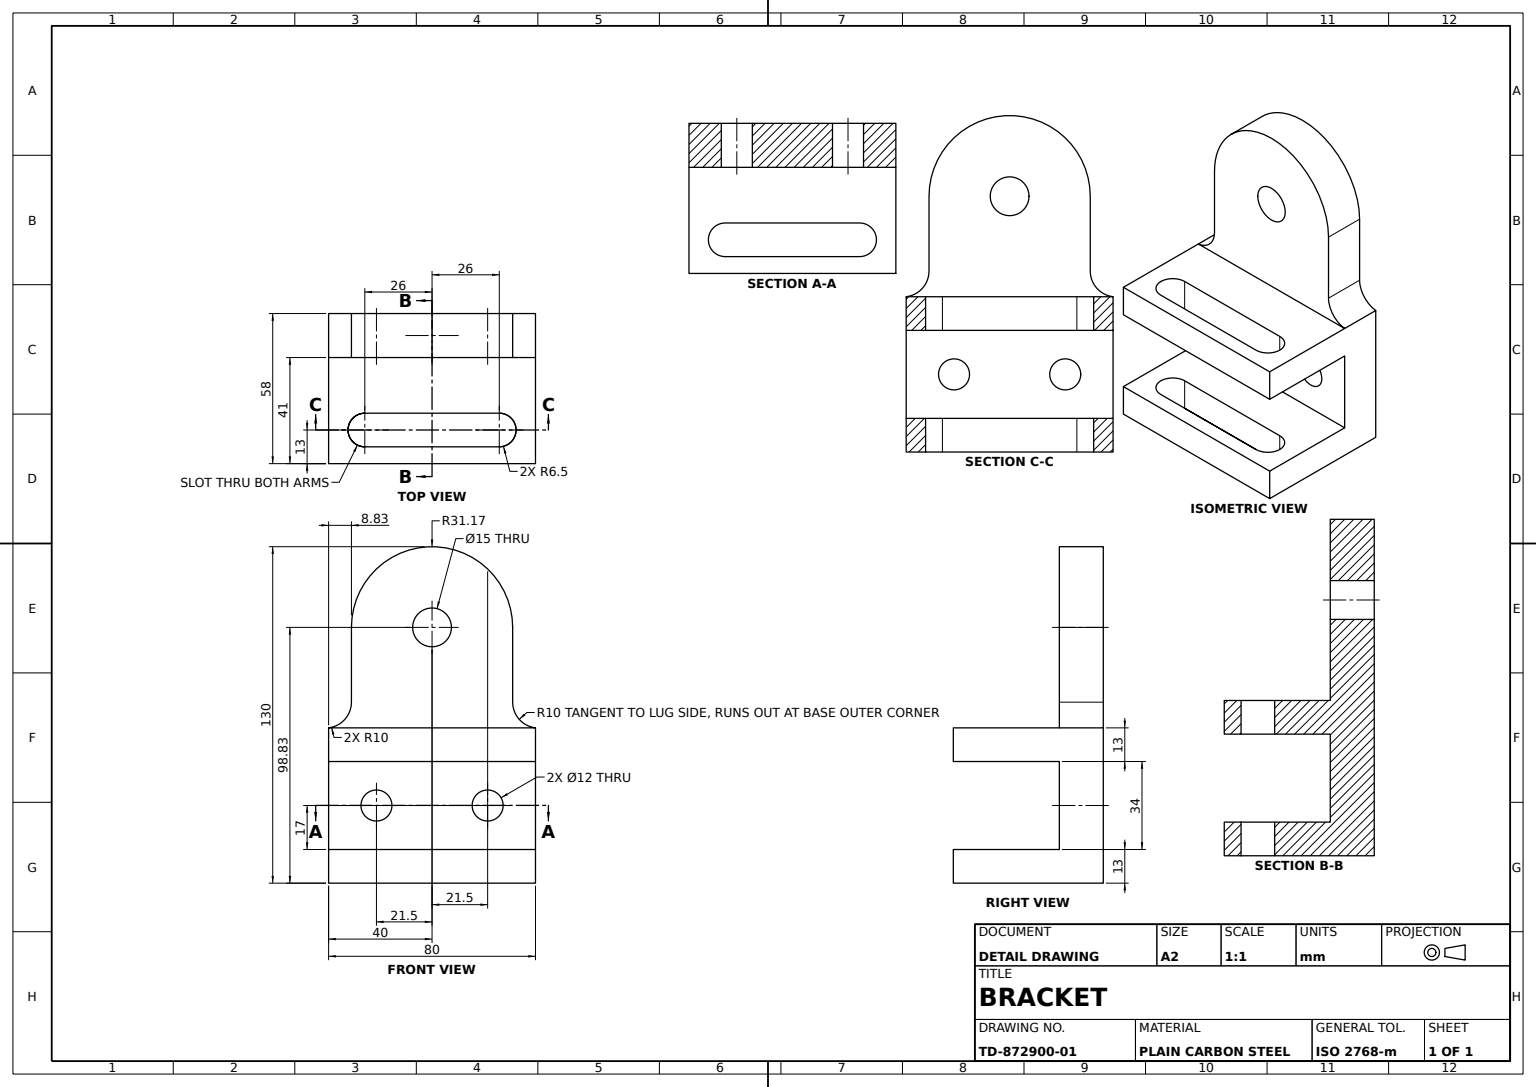
SolidWorks part; units mm, degrees
material "Plain Carbon Steel"
ref_plane "Front Plane" through (0, 0, 0) normal (0, 0, 1) x (1, 0, 0)
ref_plane "Top Plane" through (0, 0, 0) normal (0, 1, 0) x (1, 0, 0)
ref_plane "Right Plane" through (0, 0, 0) normal (1, 0, 0) x (0, 0, -1)
sketch "Bracket Profile Sketch" plane through (0, 0, 0) normal (0, 0, 1) x (1, 0, 0)
  line L0 (0, 0) -> (58, 0)
  line L1 (58, 0) -> (58, 13)
  line L2 (58, 13) -> (17, 13)
  line L3 (0, 0) -> (0, 130)
  line L4 (0, 130) -> (17, 130)
  line L5 (17, 13) -> (17, 47)
  line L6 (17, 47) -> (58, 47)
  line L7 (58, 47) -> (58, 60)
  line L8 (58, 60) -> (17, 60)
  line L9 (17, 60) -> (17, 130)
  dimension "D1" = 17
  dimension "D2" = 130
  dimension "D3" = 13
  dimension "D4" = 13
  dimension "D5" = 34
  dimension "D6" = 58
  dimension "D7" = 41
  dimension "D8" = 17
extrude "Bracket Body" add sketch "Bracket Profile Sketch" along normal mid plane 80
sketch "Lug Shape Sketch" plane through (17, 0, 0) normal (1, 0, 0) x (0, 0, -1)
  line L0 (0, 0) -> (0, 98.8253) construction
  line L1 (-31.1747, 98.8253) -> (-31.1747, 69.9308)
  line L2 (-40, 60) -> (40, 60) construction
  line L4 (-40, 60) -> (-40, 130) construction
  line L5 (-40, 60) -> (-40, 130)
  line L6 (-40, 130) -> (40, 130)
  line L7 (40, 130) -> (40, 60)
  line L10 (31.1747, 69.9308) -> (31.1747, 98.8253)
  arc A0 (31.1747, 98.8253) -> (-31.1747, 98.8253) centre (0, 98.8253) ccw
  arc A2 (-40, 60) -> (-31.1747, 69.9308) centre (-41.1747, 69.9308) ccw
  arc A4 (40, 60) -> (31.1747, 69.9308) centre (41.1747, 69.9308) cw
  line M6 (40, 60) -> (40, 130)
  line M7 (40, 130) -> (-40, 130)
  line M8 (-40, 130) -> (-40, 60)
  dimension "D2" = 10
  dimension "D3" = 50.3016
extrude "Rounded Lug Cut" cut sketch "Lug Shape Sketch" against normal blind 80 contours A4 A0 L10 M6 M7 | A2 L1 A0 L6 M8
sketch "Pin Hole Sketch" plane through (17, 0, 0) normal (1, 0, 0) x (0, 0, -1)
  circle A0 centre (0, 98.8253) radius 7.5
  dimension "D1" = 15
extrude "Pin Hole Ø15" cut sketch "Pin Hole Sketch" against normal blind 80
sketch "Fork Gap Sketch" plane through (17, 0, 0) normal (1, 0, 0) x (0, 0, -1)
  line L0 (0, 0) -> (0, 60) construction
  line L1 (-40, 60) -> (40, 60) construction
  line L4 (0, 30) -> (-21.5, 30) construction
  circle A0 centre (-21.5, 30) radius 6
  circle A1 centre (21.5, 30) radius 6
  dimension "D1" = 12
  dimension "D2" = 21.5
extrude "Fork Gap 12mm" cut sketch "Fork Gap Sketch" against normal blind 80
sketch "Arm Slots Sketch" plane through (0, 60, 0) normal (0, 1, 0) x (1, 0, 0)
  line L0 (58, 0) -> (17, 0) construction
  line L1 (58, -40) -> (58, 40) construction
  line L2 (17, -31.1747) -> (17, 31.1747) construction
  line L3 (58, 0) -> (45, 0) construction
  line L4 (45, 0) -> (45, 26) construction
  line L5 (45, -26) -> (45, 26) construction
  line L6 (38.5, -26) -> (38.5, 26)
  line L7 (51.5, -26) -> (51.5, 26)
  arc A0 (38.5, -26) -> (51.5, -26) centre (45, -26) ccw
  arc A1 (51.5, 26) -> (38.5, 26) centre (45, 26) ccw
  point P9 (45, 0)
  dimension "D1" = 6.5
  dimension "D2" = 26
  dimension "D3" = 13
extrude "Arm Slots 2x6.5" cut sketch "Arm Slots Sketch" against normal blind 80
